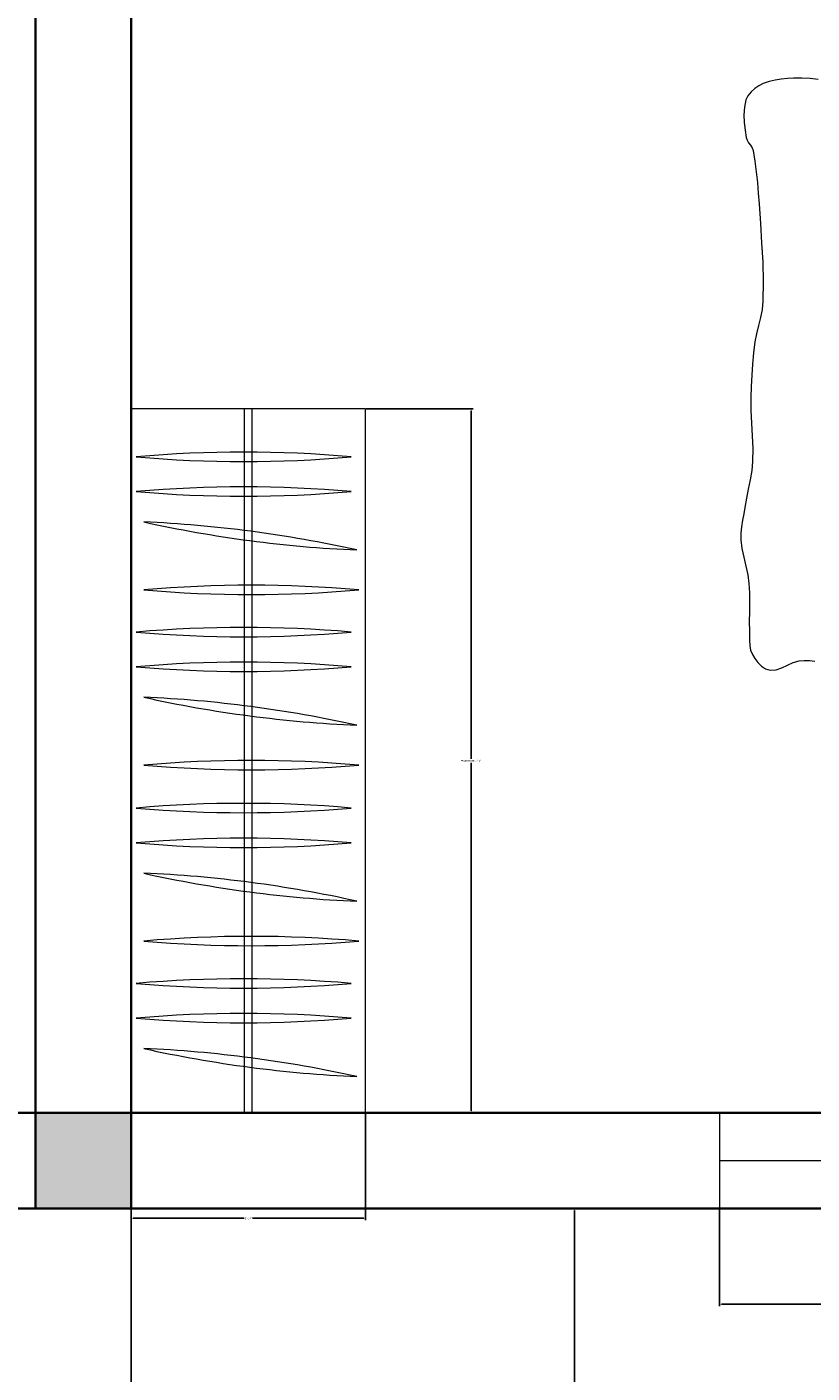
# Model space of a CAD drawing. Units: inches. Extents: x -36302355 to 648, y -221479757 to 75.
# Tile 15 of 37: x 442 to 516, y -595 to -469. Entities that reach past the tile are written whole.
import ezdxf

# ---------------------------------------------------------------- set-up
doc = ezdxf.new("R2010")
doc.units = ezdxf.units.IN
doc.header["$MEASUREMENT"] = 0
for name, color, linetype, lineweight in [('A-ANNO-DIMS', 2, 'Continuous', 18), ('A-COLS-PATT', 242, 'Continuous', 13), ('A-FLOR', 8, 'Continuous', 25), ('A-FURN', 8, 'Continuous', 13), ('A-GLAZ', 142, 'Continuous', 18), ('A-WALL', 7, 'Continuous', 35)]:
    doc.layers.add(name, color=color, linetype=linetype, lineweight=lineweight)
doc.styles.get("Standard").update_dxf_attribs({"font": 'arial.ttf'})
doc.dimstyles.get("Standard").update_dxf_attribs({"dimtxt": 0.18, "dimasz": 0.18, "dimexe": 0.18, "dimexo": 0.0625, "dimgap": 0.09, "dimtad": 0, "dimtih": 1, "dimtoh": 1, "dimdec": 0, "dimzin": 0, "dimdsep": 46, "dimlunit": 3, "dimtxsty": 'Standard', "dimcen": 0.09, "dimadec": 0, "dimazin": 0, "dimtfac": 1, "dimtdec": 0, "dimtofl": 0, "dimtmove": 0, "dimatfit": 3, "dimfxl": 1, "dimtolj": 1, "dimtzin": 0, "dimarcsym": 0})

# ---------------------------------------------------------------- blocks, each defined once
blk = doc.blocks.new('*D8')
at = {"layer": 'A-ANNO-DIMS', "color": 0, "lineweight": -2, "transparency": 16777216}
for p, q in [((495.03, -580.02), (493.69, -580.02)), ((493.87, -580.2), (493.87, -646.87)), ((493.87, -719.84), (493.87, -653.17)), ((495.03, -720.02), (493.69, -720.02))]:
    blk.add_line(p, q, dxfattribs=at)
at = {"layer": 'A-ANNO-DIMS', "color": 0, "transparency": 16777216}
for points in [[(493.84, -580.2), (493.9, -580.2), (493.87, -580.02)], [(493.84, -719.84), (493.9, -719.84), (493.87, -720.02)]]:
    blk.add_solid(points, dxfattribs=at)
at = {"layer": 'Defpoints', "color": 0, "transparency": 16777216}
for p in [(495.09, -580.02), (493.87, -720.02), (495.09, -720.02)]:
    blk.add_point(p, dxfattribs=at)
at = {"layer": 'A-ANNO-DIMS', "color": 0, "transparency": 16777216, "insert": (493.87, -650.02), "char_height": 6, "attachment_point": 5}
blk.add_mtext('\\A1;11\'-8"', dxfattribs=at)
blk = doc.blocks.new('BED-DOUBLE')
for p, q in [((0.35, 6.49), (0.31, 5.72)), ((0.42, 7.27), (0.35, 6.49)), ((55.03, 5.95), (55.04, 6.44)), ((55.04, 6.44), (55.09, 6.93)), ((0.31, 5.72), (0.32, 4.95)), ((55.07, 5.46), (55.03, 5.95)), ((55.22, 4.91), (55.07, 5.46)), ((0.32, 4.95), (0.35, 4.37)), ((0.35, 4.37), (0.4, 3.78)), ((55.47, 4.37), (55.22, 4.91)), ((55.73, 3.84), (55.47, 4.37)), ((55.91, 3.3), (55.73, 3.84)), ((0.4, 3.78), (0.49, 3.21)), ((0.49, 3.21), (0.62, 2.64)), ((0.62, 2.64), (0.82, 2.1)), ((55.81, 2.32), (55.94, 2.75)), ((55.94, 2.75), (55.91, 3.3)), ((0.82, 2.1), (1.03, 1.69)), ((1.03, 1.69), (1.29, 1.3)), ((1.29, 1.3), (1.59, 0.95)), ((7.11, 1.14), (8.1, 1.31)), ((8.1, 1.31), (9.1, 1.44)), ((9.1, 1.44), (10.11, 1.55)), ((10.11, 1.55), (11.12, 1.63)), ((11.12, 1.63), (12.12, 1.7)), ((12.12, 1.7), (13.95, 1.82)), ((13.95, 1.82), (15.78, 1.94)), ((15.78, 1.94), (17.61, 2.04)), ((17.61, 2.04), (19.43, 2.09)), ((19.43, 2.09), (21.26, 2.07)), ((21.26, 2.07), (22.04, 2)), ((22.04, 2), (22.8, 1.84)), ((22.8, 1.84), (23.56, 1.64)), ((23.56, 1.64), (24.32, 1.45)), ((24.32, 1.45), (25.08, 1.31)), ((25.08, 1.31), (26.13, 1.19)), ((54.46, 1.07), (54.86, 1.31)), ((54.86, 1.31), (55.24, 1.6)), ((55.24, 1.6), (55.57, 1.94)), ((55.57, 1.94), (55.81, 2.32)), ((1.59, 0.95), (1.95, 0.66)), ((1.95, 0.66), (2.35, 0.47)), ((2.35, 0.47), (3.04, 0.32)), ((3.04, 0.32), (3.74, 0.27)), ((3.74, 0.27), (4.46, 0.31)), ((4.46, 0.31), (5.18, 0.39)), ((5.18, 0.39), (5.89, 0.49)), ((5.89, 0.49), (6.14, 0.57)), ((6.14, 0.57), (6.38, 0.72)), ((6.38, 0.72), (6.61, 0.89)), ((6.61, 0.89), (6.85, 1.05)), ((6.85, 1.05), (7.11, 1.14)), ((26.13, 1.19), (27.18, 1.09)), ((27.18, 1.09), (28.23, 1.01)), ((28.23, 1.01), (29.28, 0.95)), ((29.28, 0.95), (30.33, 0.92)), ((30.33, 0.92), (31.53, 0.93)), ((31.53, 0.93), (32.73, 0.99)), ((32.73, 0.99), (33.92, 1.06)), ((33.92, 1.06), (35.12, 1.11)), ((35.12, 1.11), (36.32, 1.09)), ((36.32, 1.09), (37.19, 1.01)), ((37.19, 1.01), (38.06, 0.86)), ((38.06, 0.86), (38.92, 0.69)), ((38.92, 0.69), (39.78, 0.51)), ((39.78, 0.51), (40.65, 0.36)), ((40.65, 0.36), (41.25, 0.26)), ((41.25, 0.26), (41.86, 0.15)), ((41.86, 0.15), (42.47, 0.06)), ((42.47, 0.06), (43.08, 0)), ((43.08, 0), (43.7, 0)), ((43.7, 0), (44.52, 0.09)), ((44.52, 0.09), (45.34, 0.26)), ((45.34, 0.26), (46.16, 0.45)), ((46.16, 0.45), (46.98, 0.63)), ((46.98, 0.63), (47.8, 0.75)), ((47.8, 0.75), (48.69, 0.8)), ((48.69, 0.8), (49.59, 0.81)), ((49.59, 0.81), (50.48, 0.79)), ((50.48, 0.79), (51.38, 0.78)), ((51.38, 0.78), (52.27, 0.8)), ((52.27, 0.8), (52.72, 0.81)), ((52.72, 0.81), (53.17, 0.81)), ((53.17, 0.81), (53.62, 0.83)), ((53.62, 0.83), (54.06, 0.91)), ((54.06, 0.91), (54.46, 1.07))]:
    blk.add_line(p, q)
blk = doc.blocks.new('WARDROBE-HANGING')
for p, q in [((0, 0), (0, 53.32)), ((17.77, 53.32), (0, 53.32)), ((8.59, 0), (8.59, 53.32)), ((9.18, 0), (9.18, 53.32)), ((17.77, 0), (17.77, 53.32)), ((17.77, 0), (0, 0))]:
    blk.add_line(p, q)
for centre, start, end in [((8.53, -43.46), 85.0028, 94.9972), ((8.53, 142.85), 265.0028, 274.9972), ((8.53, -46.09), 85.0028, 94.9972), ((8.53, 140.22), 265.0028, 274.9972), ((21.18, 136.06), 257.508, 267.5023), ((-3.12, -48.66), 77.508, 87.5023), ((9.1, -53.54), 85.0028, 94.9972), ((9.1, 132.77), 265.0028, 274.9972), ((8.53, -56.74), 85.0028, 94.9972), ((8.53, 129.57), 265.0028, 274.9972), ((8.53, -59.37), 85.0028, 94.9972), ((8.53, 126.94), 265.0028, 274.9972), ((21.18, 122.78), 257.508, 267.5023), ((-3.12, -61.94), 77.508, 87.5023), ((9.1, -66.82), 85.0028, 94.9972), ((9.1, 119.49), 265.0028, 274.9972), ((8.53, -70.07), 85.0028, 94.9972), ((8.53, 116.24), 265.0028, 274.9972), ((8.53, -72.71), 85.0028, 94.9972), ((8.53, 113.6), 265.0028, 274.9972), ((-3.12, -75.27), 77.508, 87.5023), ((21.18, 109.44), 257.508, 267.5023), ((9.1, -80.15), 85.0028, 94.9972), ((9.1, 106.16), 265.0028, 274.9972), ((8.53, -83.36), 85.0028, 94.9972), ((8.53, 102.95), 265.0028, 274.9972), ((8.53, -85.99), 85.0028, 94.9972), ((8.53, 100.32), 265.0028, 274.9972), ((-3.12, -88.56), 77.508, 87.5023), ((21.18, 96.16), 257.508, 267.5023)]:
    blk.add_arc(centre, 93.51, start, end)
blk = doc.blocks.new('WIN-60')
for p, q in [((60, 9), (0, 9)), ((0, 9), (0, 0)), ((60, 0), (60, 9)), ((0, 4.5), (60, 4.5)), ((0, 0), (60, 0))]:
    blk.add_line(p, q)
blk = doc.blocks.new('*D23')
at = {"layer": 'A-ANNO-DIMS', "color": 0, "lineweight": -2, "transparency": 16777216}
for p, q in [((507.51, -580.08), (507.51, -589.2)), ((567.51, -580.08), (567.51, -589.2)), ((507.69, -589.02), (536.28, -589.02)), ((567.33, -589.02), (538.74, -589.02))]:
    blk.add_line(p, q, dxfattribs=at)
at = {"layer": 'A-ANNO-DIMS', "color": 0, "transparency": 16777216}
for points in [[(507.69, -588.99), (507.69, -589.05), (507.51, -589.02)], [(567.33, -588.99), (567.33, -589.05), (567.51, -589.02)]]:
    blk.add_solid(points, dxfattribs=at)
at = {"layer": 'Defpoints', "color": 0, "transparency": 16777216}
for p in [(507.51, -580.02), (567.51, -580.02), (567.51, -589.02)]:
    blk.add_point(p, dxfattribs=at)
at = {"layer": 'A-ANNO-DIMS', "color": 0, "transparency": 16777216, "insert": (537.51, -589.02), "char_height": 0.18, "attachment_point": 5}
blk.add_mtext('\\A1;WINDOW 5\'-0" TYP.', dxfattribs=at)
blk = doc.blocks.new('*D47')
at = {"layer": 'A-ANNO-DIMS', "color": 0, "lineweight": -2, "transparency": 16777216}
for p, q in [((474.3, -504.88), (484.34, -504.88)), ((484.16, -505.06), (484.16, -537.77)), ((484.16, -570.84), (484.16, -538.13)), ((474.3, -571.02), (484.34, -571.02))]:
    blk.add_line(p, q, dxfattribs=at)
at = {"layer": 'A-ANNO-DIMS', "color": 0, "transparency": 16777216}
for points in [[(484.13, -505.06), (484.19, -505.06), (484.16, -504.88)], [(484.13, -570.84), (484.19, -570.84), (484.16, -571.02)]]:
    blk.add_solid(points, dxfattribs=at)
at = {"layer": 'Defpoints', "color": 0, "transparency": 16777216}
for p in [(474.24, -504.88), (484.16, -504.88), (474.24, -571.02)]:
    blk.add_point(p, dxfattribs=at)
at = {"layer": 'A-ANNO-DIMS', "color": 0, "transparency": 16777216, "insert": (484.16, -537.95), "char_height": 0.18, "attachment_point": 5}
blk.add_mtext('\\A1;WARDROBE 5\'-6"', dxfattribs=at)
blk = doc.blocks.new('*D48')
at = {"layer": 'A-ANNO-DIMS', "color": 0, "lineweight": -2, "transparency": 16777216}
for p, q in [((452.2, -571.08), (452.2, -581.12)), ((474.24, -571.08), (474.24, -581.12)), ((452.38, -580.94), (462.83, -580.94)), ((474.06, -580.94), (463.61, -580.94))]:
    blk.add_line(p, q, dxfattribs=at)
at = {"layer": 'A-ANNO-DIMS', "color": 0, "transparency": 16777216}
for points in [[(452.38, -580.91), (452.38, -580.97), (452.2, -580.94)], [(474.06, -580.91), (474.06, -580.97), (474.24, -580.94)]]:
    blk.add_solid(points, dxfattribs=at)
at = {"layer": 'Defpoints', "color": 0, "transparency": 16777216}
for p in [(452.2, -571.02), (474.24, -571.02), (474.24, -580.94)]:
    blk.add_point(p, dxfattribs=at)
at = {"layer": 'A-ANNO-DIMS', "color": 0, "transparency": 16777216, "insert": (463.22, -580.94), "char_height": 0.18, "attachment_point": 5}
blk.add_mtext('\\A1;1\'-10"', dxfattribs=at)

msp = doc.modelspace()

# ---------------------------------------------------------------- hatches: boundary and pattern name
at = {"layer": 'A-COLS-PATT'}
h = msp.add_hatch(color=256, dxfattribs=at)
h.dxf.hatch_style = 1
h.paths.add_polyline_path([(145.2, 24.98), (145.2, 15.98), (154.2, 15.98), (154.2, 24.98)])
h.paths.add_polyline_path([(247.2, 15.98), (247.2, 24.98), (238.2, 24.98), (238.2, 15.98)])
h.paths.add_polyline_path([(387.64, 15.98), (395.7, 15.98), (395.7, 24.98), (387.64, 24.98)])
h.paths.add_polyline_path([(451.26, 24.98), (443.7, 24.98), (443.7, 15.98), (451.26, 15.98)])
h.paths.add_polyline_path([(596.2, 15.98), (605.2, 15.98), (605.2, 24.98), (596.2, 24.98)])
h.paths.add_polyline_path([(238.2, -122.02), (238.2, -131.02), (247.2, -131.02), (247.2, -122.02)])
h.paths.add_polyline_path([(395.7, -122.02), (387.46, -122.02), (387.46, -131.02), (395.7, -131.02)])
h.paths.add_polyline_path([(448.2, -131.02), (453.73, -131.02), (453.73, -122.02), (443.7, -122.02), (443.7, -131.02)])
h.paths.add_polyline_path([(596.2, -131.02), (605.2, -131.02), (605.2, -122.02), (596.2, -122.02)])
h.paths.add_polyline_path([(145.2, -176.97), (154.2, -176.97), (154.2, -167.02), (145.2, -167.02)])
h.paths.add_polyline_path([(314.2, -176.97), (323.2, -176.97), (323.2, -167.02), (314.2, -167.02)])
h.paths.add_polyline_path([(154.2, -314.02), (154.2, -309.52), (145.2, -309.52), (145.2, -314.02)])
h.paths.add_polyline_path([(314.2, -309.52), (314.2, -318.52), (323.2, -318.52), (323.2, -309.52)])
h.paths.add_polyline_path([(448.2, -277.02), (443.7, -277.02), (443.7, -286.02), (448.2, -286.02)])
h.paths.add_polyline_path([(283.2, -370.02), (274.2, -370.02), (274.2, -379.02), (283.2, -379.02), (283.2, -374.52)])
h.paths.add_polyline_path([(154.2, -370.02), (145.2, -370.02), (145.2, -379.02), (154.2, -379.02)])
h.paths.add_polyline_path([(443.2, -374.52), (443.2, -379.02), (452.2, -379.02), (452.2, -374.52)])
h.paths.add_polyline_path([(145.2, -580.02), (154.2, -580.02), (154.2, -571.02), (145.2, -571.02)])
h.paths.add_polyline_path([(274.2, -571.02), (274.2, -580.02), (283.2, -580.02), (283.2, -571.02)])
h.paths.add_polyline_path([(443.2, -580.02), (452.2, -580.02), (452.2, -571.02), (443.2, -571.02)])

# ---------------------------------------------------------------- linework, layer by layer
at = {"layer": 'A-FLOR'}
msp.add_line((452.2, -580.02), (452.2, -651.02), dxfattribs=at)
at = {"layer": 'A-WALL'}
for p, q in [((443.2, -374.52), (443.2, -580.02)), ((452.2, -374.52), (452.2, -580.02)), ((335.2, -571.02), (605.2, -571.02)), ((335.2, -580.02), (605.2, -580.02))]:
    msp.add_line(p, q, dxfattribs=at)

# ---------------------------------------------------------------- block references
at = {"layer": 'A-FURN', "rotation": 270}
msp.add_blockref('BED-DOUBLE', (509.53, -473.48), dxfattribs=at)
at = {"layer": 'A-FURN', "xscale": 1.240462180178274, "yscale": 1.240462180178274, "rotation": 8.537736463e-07}
msp.add_blockref('WARDROBE-HANGING', (452.2, -571.02), dxfattribs=at)
at = {"layer": 'A-GLAZ'}
msp.add_blockref('WIN-60', (507.51, -580.02), dxfattribs=at)

# ---------------------------------------------------------------- dimensions: what is measured, and where the dimension line sits
at = {"layer": 'A-ANNO-DIMS'}
dim = msp.add_linear_dim(base=(484.16, -504.88), p1=(474.24, -571.02), p2=(474.24, -504.88), angle=90, text='WARDROBE <>', dimstyle='Standard', override={"dimdec": 1, "dimlfac": 1, "dimrnd": 0, "dimzin": 1, "dimdsep": 46, "dimlunit": 4, "dimfrac": 2}, dxfattribs=at)
dim.commit()
dim.dimension.update_dxf_attribs({"geometry": '*D47', "text_midpoint": (484.16, -537.95)})
for base, p1, p2, angle, override, picture, middle in [((474.24, -580.94), (452.2, -571.02), (474.24, -571.02), 0, {"dimdec": 1, "dimlfac": 1, "dimrnd": 0, "dimzin": 1, "dimdsep": 46, "dimlunit": 4, "dimfrac": 2}, '*D48', (463.22, -580.94)), ((493.87, -720.02), (495.09, -580.02), (495.09, -720.02), 90, {"dimtxt": 6, "dimclrd": 0, "dimclre": 0, "dimclrt": 0}, '*D8', (493.87, -650.02))]:
    dim = msp.add_linear_dim(base=base, p1=p1, p2=p2, angle=angle, dimstyle='Standard', override=override, dxfattribs=at)
    dim.commit()
    dim.dimension.update_dxf_attribs({"geometry": picture, "text_midpoint": middle})
dim = msp.add_linear_dim(base=(567.51, -589.02), p1=(507.51, -580.02), p2=(567.51, -580.02), text='WINDOW <> TYP.', dimstyle='Standard', override={"dimdec": 1, "dimlfac": 1, "dimrnd": 0, "dimzin": 1, "dimdsep": 46, "dimlunit": 4, "dimfrac": 2}, dxfattribs=at)
dim.commit()
dim.dimension.update_dxf_attribs({"geometry": '*D23', "text_midpoint": (537.51, -589.02)})

doc.saveas('drawing.dxf')
